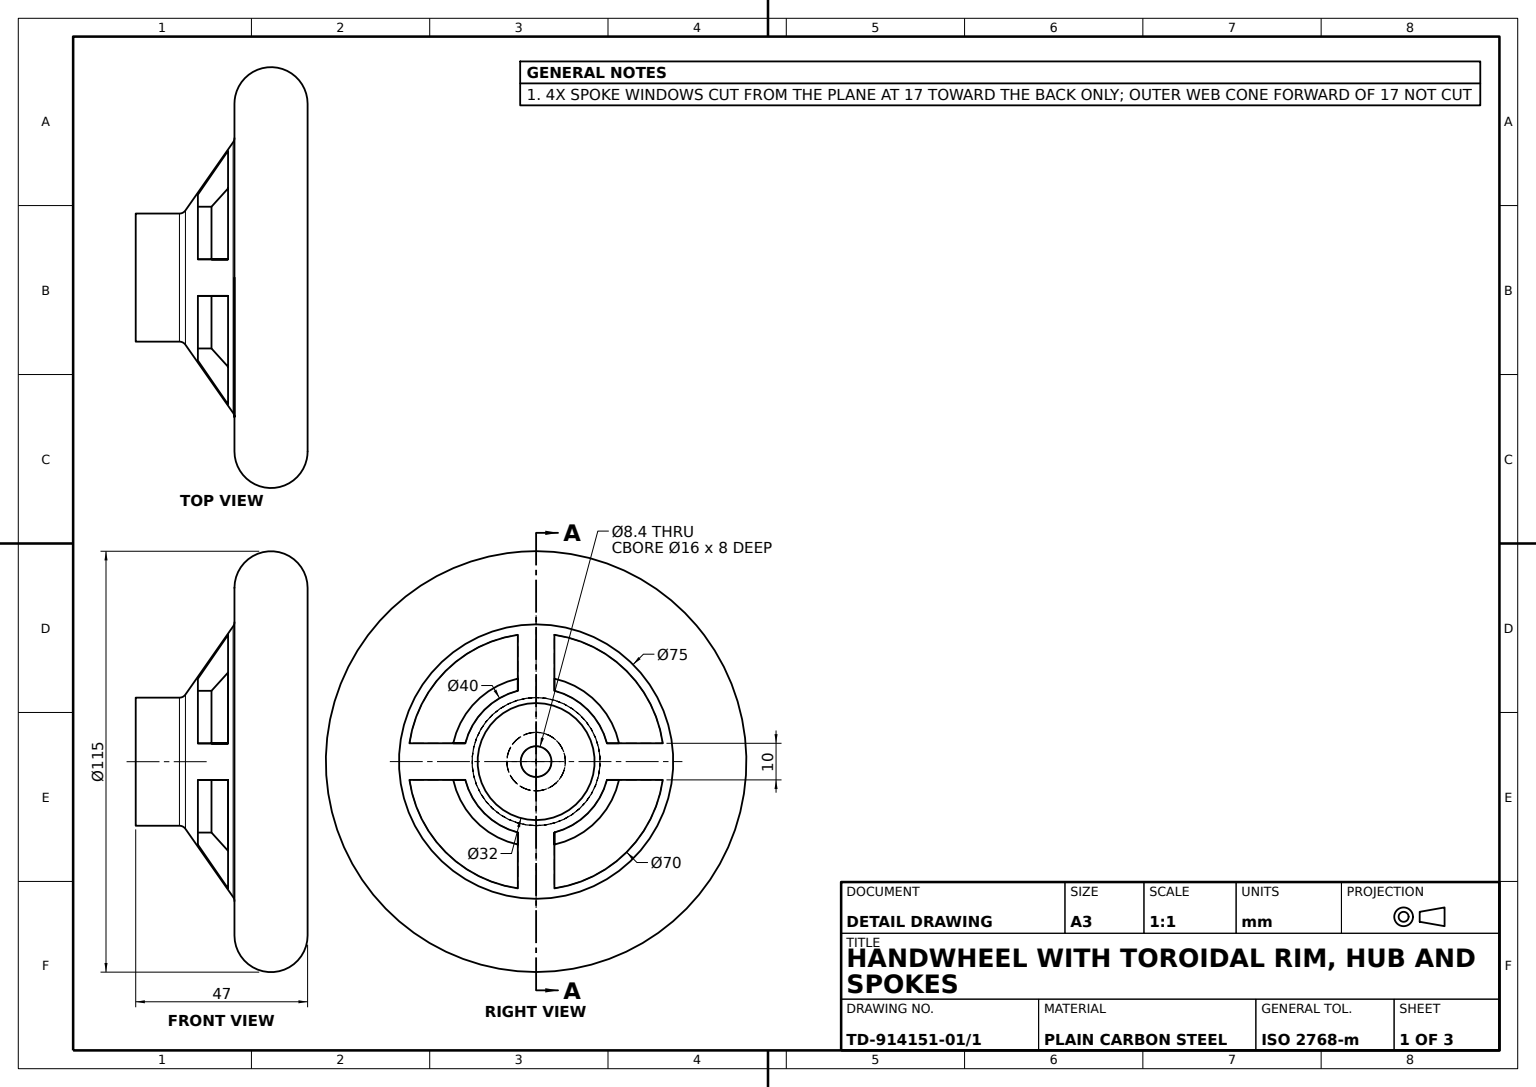
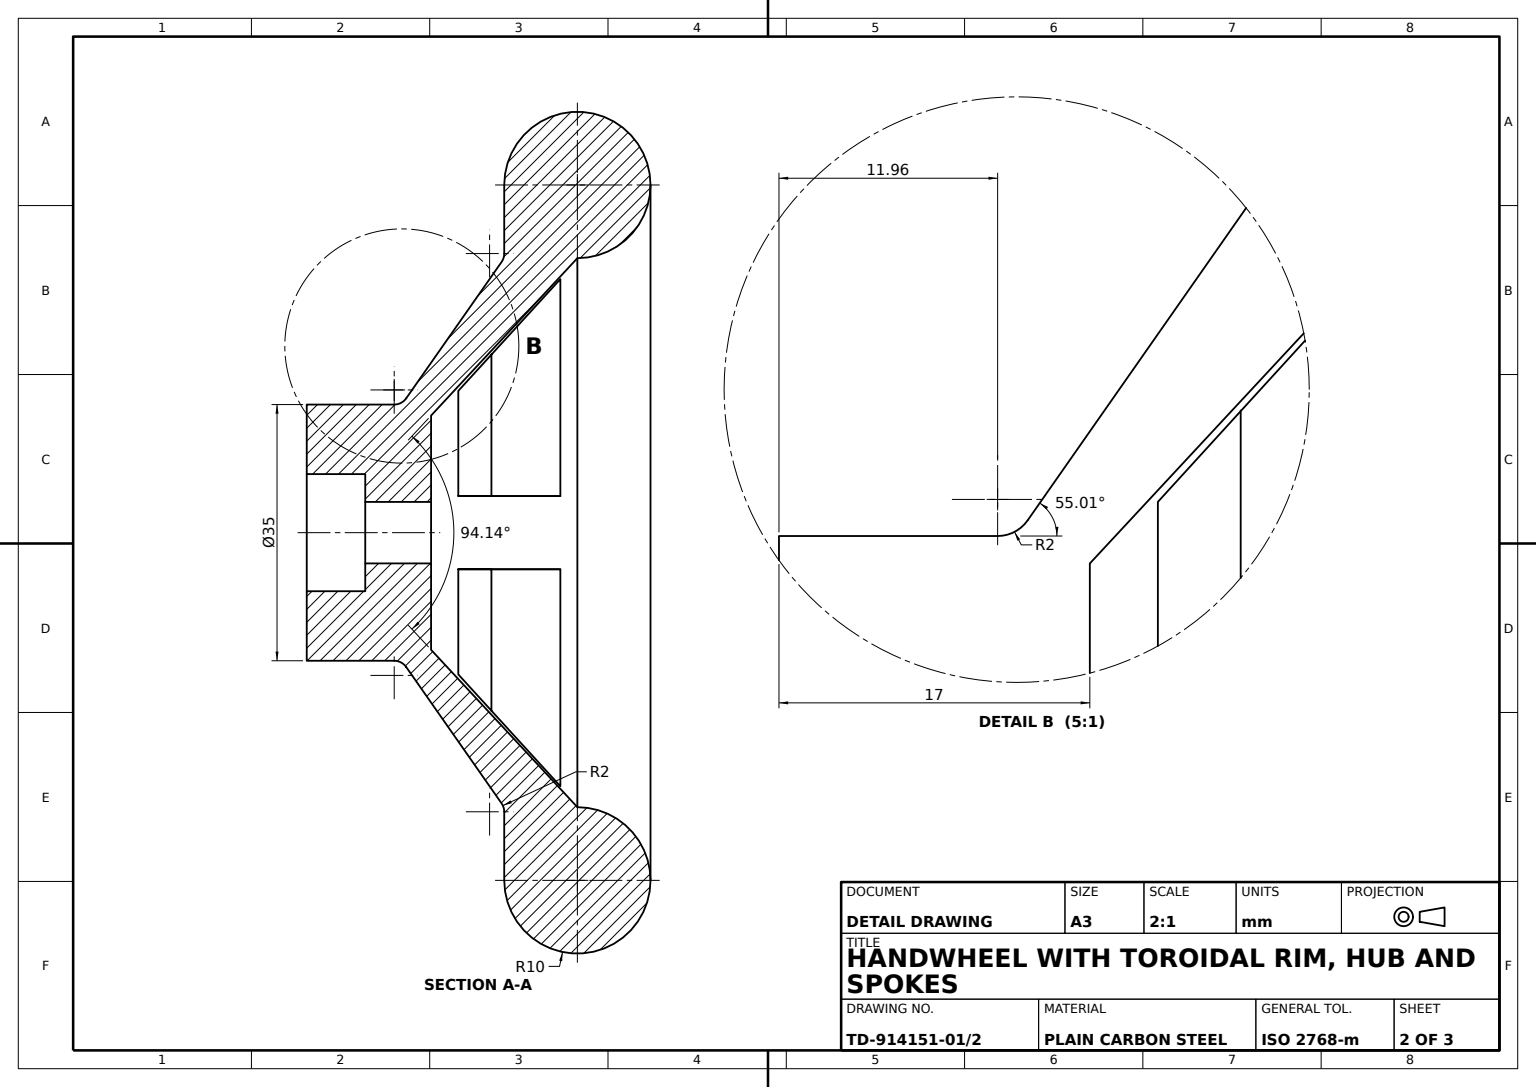
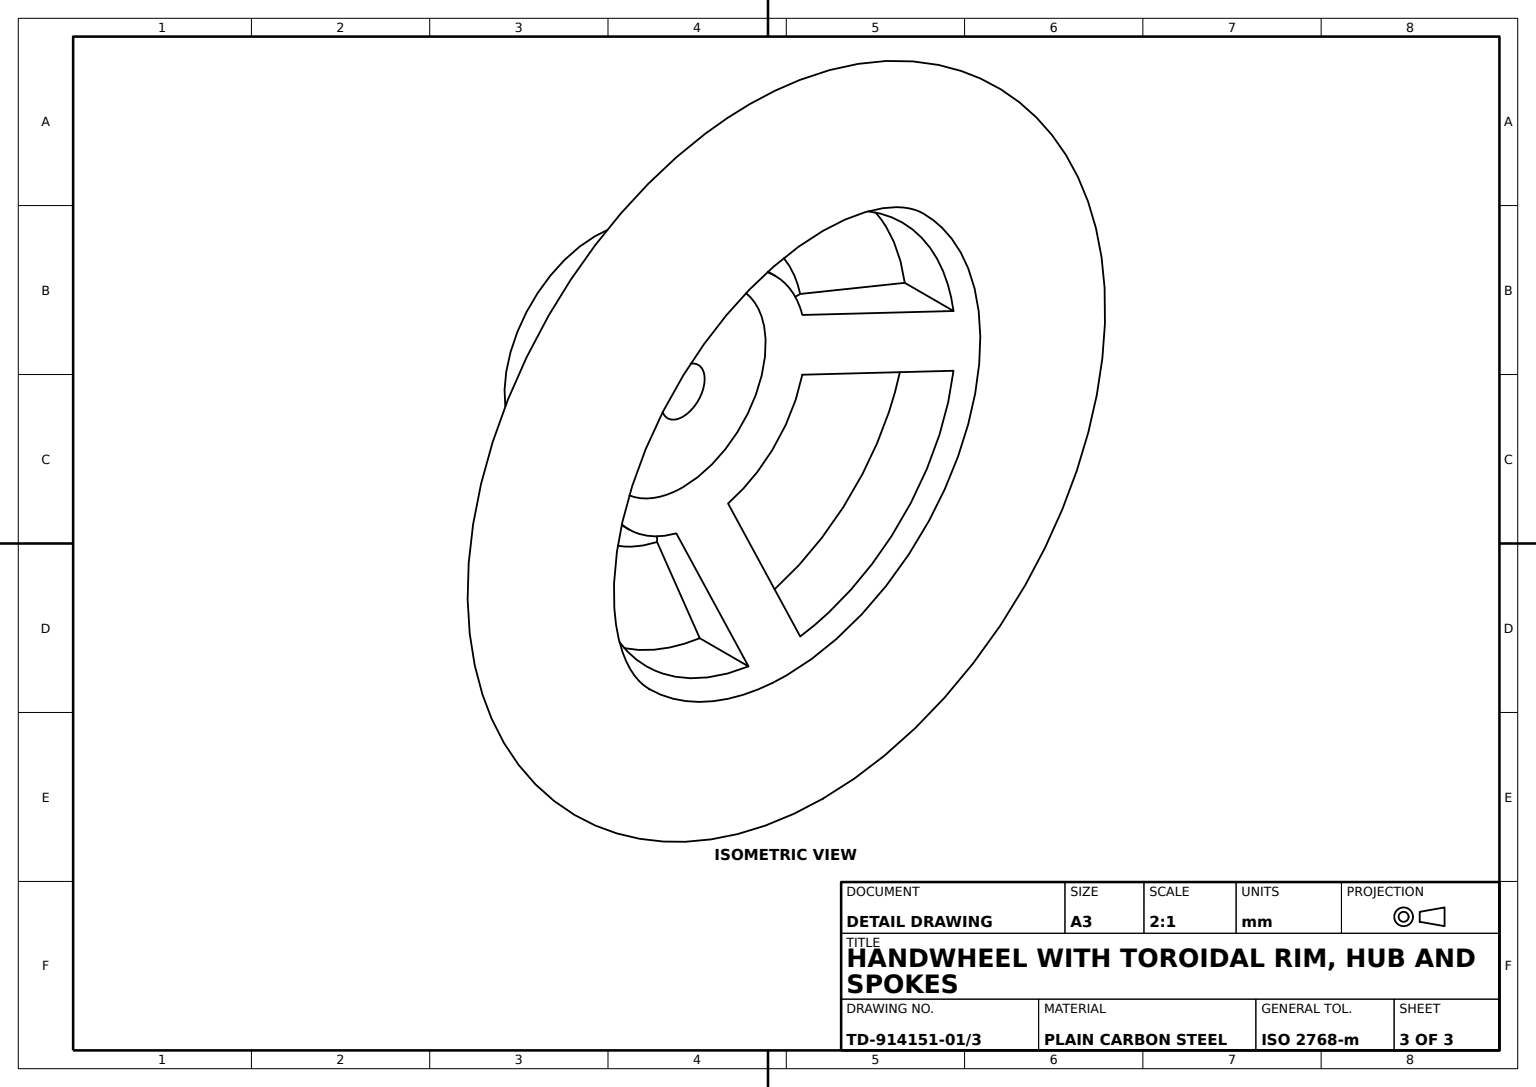
from build123d import *

# Parameters (mm, degrees)
SPOKE_WINDOWS_4X_DEPTH = 20


with BuildPart() as part:
    # Handwheel Profile Sketch → Handwheel Body (revolve)
    with BuildSketch(Plane.XY):
        with BuildLine():
            Line((-8, -37), (-17.5, -37))
            Line((-17.5, -37), (-17.5, -25.041311123))
            ThreePointArc((-17.5, -25.041311123), (-17.726042647, -24.117690362), (-18.353075311, -23.402847282))
            Line((-18.353075311, -23.402847282), (-36.983519773, -10.361536159))
            ThreePointArc((-36.983519773, -10.361536159), (-37.529165692, -10.092524223), (-38.130444462, -10))
            Line((-38.130444462, -10), (-47.5, -10))
            ThreePointArc((-47.5, -10), (-54.571067812, 7.071067812), (-37.5, 0))
            Line((-37.5, 0), (-16, -20))
            Line((-16, -20), (-4.2, -20))
            Line((-4.2, -20), (-4.2, -29))
            Line((-4.2, -29), (-8, -29))
            Line((-8, -29), (-8, -37))
        make_face()
    revolve(axis=Axis((0, 48.530715578, 0), (0, -1, 0)))

    # Spoke Windows Sketch → Spoke Windows 4x (cut)
    with BuildSketch(Plane(origin=(0, -20, 0), x_dir=(1, 0, 0), z_dir=(0, 1, 0))):
        with BuildLine():
            Line((19.364916731, 5), (34.641016151, 5))
            ThreePointArc((34.641016151, 5), (24.748737342, 24.748737342), (5, 34.641016151))
            Line((5, 34.641016151), (5, 19.364916731))
            ThreePointArc((5, 19.364916731), (14.142135624, 14.142135624), (19.364916731, 5))
        make_face()
        with BuildLine():
            Line((34.641016151, -5), (19.364916731, -5))
            ThreePointArc((19.364916731, -5), (14.142135624, -14.142135624), (5, -19.364916731))
            Line((5, -19.364916731), (5, -34.641016151))
            ThreePointArc((5, -34.641016151), (24.748737342, -24.748737342), (34.641016151, -5))
        make_face()
        with BuildLine():
            ThreePointArc((-5, 34.641016151), (-24.748737342, 24.748737342), (-34.641016151, 5))
            Line((-34.641016151, 5), (-19.364916731, 5))
            ThreePointArc((-19.364916731, 5), (-14.142135624, 14.142135624), (-5, 19.364916731))
            Line((-5, 19.364916731), (-5, 34.641016151))
        make_face()
        with BuildLine():
            ThreePointArc((-34.641016151, -5), (-24.748737342, -24.748737342), (-5, -34.641016151))
            Line((-5, -34.641016151), (-5, -19.364916731))
            ThreePointArc((-5, -19.364916731), (-14.142135624, -14.142135624), (-19.364916731, -5))
            Line((-19.364916731, -5), (-34.641016151, -5))
        make_face()
    extrude(amount=SPOKE_WINDOWS_4X_DEPTH, mode=Mode.SUBTRACT)


solid = part.part
